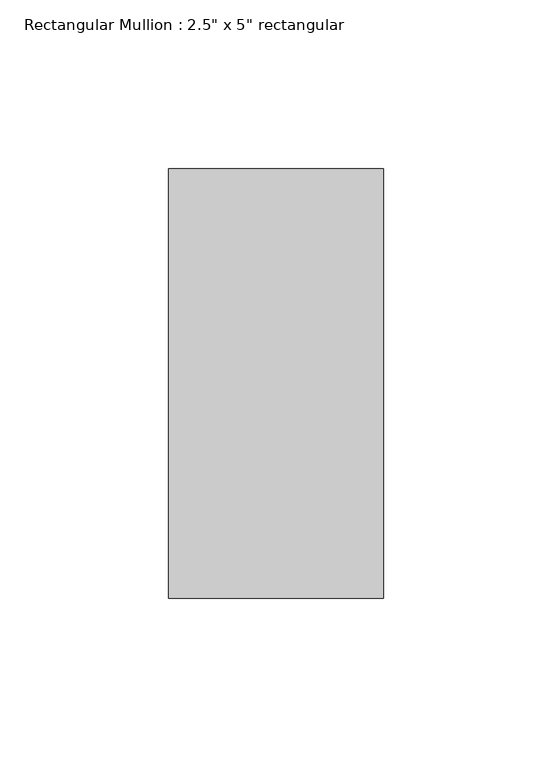
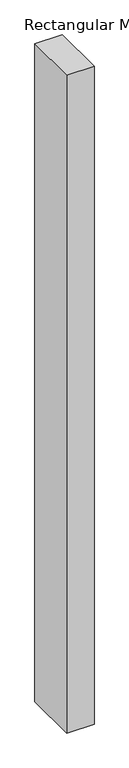
"""IFC4 building model written with IfcOpenShell, lengths in millimetres: member geometry."""

from ifc_helpers import new_model, si_unit, frame, origin, place, context, project, spatial, polyline, outline, extrude, source, transform, mapped, element, save


def member_5bd926c3(model_context):
    return source(origin(), model_context, "Body", "SweptSolid", [
        extrude(outline(polyline([(0.0, 63.5), (0.0, -63.5), (-63.5, -63.5), (-63.5, 63.5), (0.0, 63.5)])), frame((0.0, 0.0, -1609.522501), z_axis=(0.0, 0.0, 1.0), x_axis=(1.0, 0.0, 0.0)), (0.0, 0.0, 1.0), 1609.522501),
    ])


if __name__ == "__main__":
    model = new_model("IFC4")
    model_context = context("Model", 3, world=origin())
    ifc_project = project(units=[si_unit("LENGTHUNIT", "METRE", prefix="MILLI")], contexts=[model_context])
    site = spatial("IfcSite", under=ifc_project)
    building = spatial("IfcBuilding", under=site)
    placement = place(None, origin())
    member_shape = member_5bd926c3(model_context)
    element("IfcMember", 1, ObjectType="Rectangular Mullion : 2.5\" x 5\" rectangular", at=placement, inside=building, context=model_context, shape_type="MappedRepresentation", body=[
        mapped(member_shape, transform((0.0, 0.0, 0.0), x_axis=(1.0, 0.0, 0.0), y_axis=(0.0, 1.0, 0.0), z_axis=(0.0, 0.0, 1.0))),
    ])
    save(model, "model.ifc")

# Revit data of these elements
# Type "Rectangular Mullion : 2.5\" x 5\" rectangular"
#   built-in parameter 1007304 = 0.416667 (stored number, unit not read)
#   built-in parameter 1007301 = 0.104167 (stored number, unit not read)
#   built-in parameter 1007300 = 0.104167 (stored number, unit not read)
# Element 1 (IfcMember, "Rectangular Mullion : 2.5\" x 5\" rectangular")
#   Materials on its faces: "Aluminum"
# Materials
#   "Aluminum": class "Metal", colour RGB 247 247 247, transparency 0, Description = "Aluminum 6061", Cost = 0
